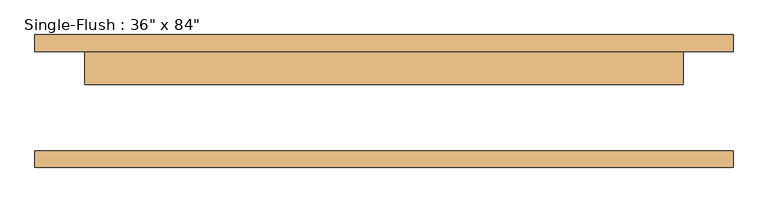
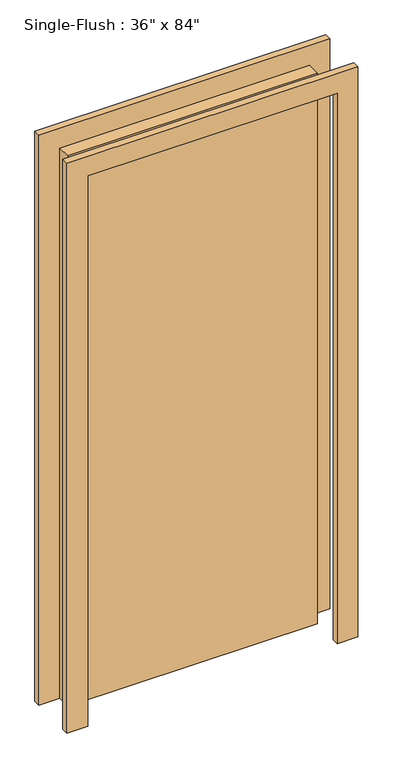
"""IFC4 building model written with IfcOpenShell, lengths in millimetres: door geometry."""

from ifc_helpers import new_model, si_unit, frame, origin, origin_with_axes, place, context, project, spatial, polyline, outline, extrude, source, transform, mapped, element, save


def door_16372e1c(model_context):
    return source(origin(), model_context, "Body", "SweptSolid", [
        extrude(outline(polyline([(2209.8, -533.4), (0.0, -533.4), (0.0, -457.2), (2133.6, -457.2), (2133.6, 457.2), (0.0, 457.2), (0.0, 533.4), (2209.8, 533.4), (2209.8, -533.4)])), frame((0.0, 76.2, 0.0), z_axis=(0.0, 1.0, 0.0), x_axis=(0.0, 0.0, 1.0)), (0.0, 0.0, 1.0), 25.4),
        extrude(outline(polyline([(2209.8, 533.4), (2209.8, -533.4), (0.0, -533.4), (0.0, -457.2), (2133.6, -457.2), (2133.6, 457.2), (0.0, 457.2), (0.0, 533.4), (2209.8, 533.4)])), frame((0.0, -101.6, 0.0), z_axis=(0.0, 1.0, 0.0), x_axis=(0.0, 0.0, 1.0)), (0.0, 0.0, 1.0), 25.4),
        extrude(outline(polyline([(457.2, 25.4), (-457.2, 25.4), (-457.2, 76.2), (457.2, 76.2), (457.2, 25.4)])), origin_with_axes(), (0.0, 0.0, 1.0), 2133.6),
    ])


if __name__ == "__main__":
    model = new_model("IFC4")
    model_context = context("Model", 3, world=origin())
    ifc_project = project(units=[si_unit("LENGTHUNIT", "METRE", prefix="MILLI")], contexts=[model_context])
    site = spatial("IfcSite", under=ifc_project)
    building = spatial("IfcBuilding", under=site)
    placement = place(None, origin())
    door_shape = door_16372e1c(model_context)
    element("IfcDoor", 1, ObjectType="Single-Flush : 36\" x 84\"", at=placement, inside=building, context=model_context, shape_type="MappedRepresentation", body=[
        mapped(door_shape, transform((0.0, 0.0, 0.0), x_axis=(1.0, 0.0, 0.0), y_axis=(0.0, 1.0, 0.0), z_axis=(0.0, 0.0, 1.0))),
    ])
    save(model, "model.ifc")

# Revit data of these elements
# Type "Single-Flush : 36\" x 84\""
#   Type Mark = "1"
#   Construction Type Id = "MDOOR"
#   Assembly Code = "C1020"
#   Analytic Construction = "Metal"
#   Thickness = 0' - 2"
#   Heat Transfer Coefficient (U) = 0.651978 BTU/(h·ft²·°F)
#   Height = 7' - 0"
#   Trim Projection Ext = 0' - 1"
#   Trim Projection Int = 0' - 1"
#   Trim Width = 0' - 3"
#   Width = 3' - 0"
#   Define Thermal Properties by = 1
#   Define Thermal Properties by = 1
#   Door Material = Door - Panel
#   Frame Material = Door - Frame
#   Visual Light Transmittance = 0
#   Solar Heat Gain Coefficient = 0
#   Function = (empty or 0)
#   Wall Closure = (empty or 0)
# Element 1 (IfcDoor, "Single-Flush : 36\" x 84\"")
#   Materials on its faces: "Door - Frame", "Door - Panel"
# Materials
#   "Door - Panel": class "Wood", colour RGB 210 159 95, transparency 0, Cost = 0
#   "Door - Frame": colour RGB 118 70 51, transparency 0, Cost = 0
